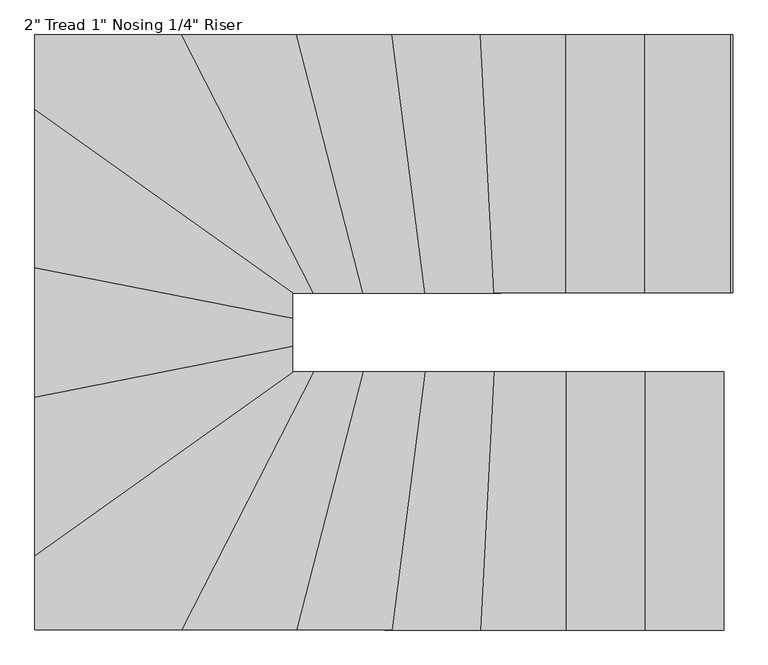
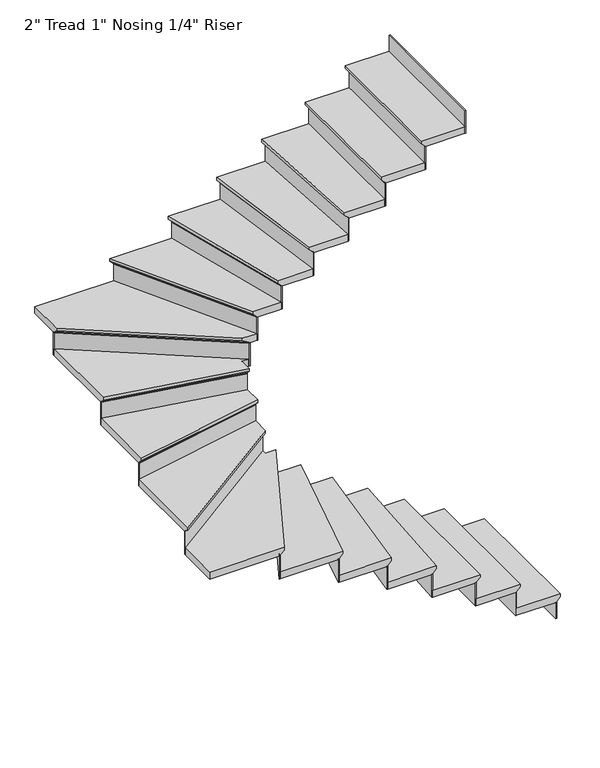
"""IFC4 building model written with IfcOpenShell, lengths in millimetres: stair flight geometry."""

from ifc_helpers import new_model, si_unit, origin, place, context, project, spatial, faceted_brep, source, transform, mapped, element, save


def stair_flight_62da4333(model_context):
    return source(origin(), model_context, "Body", "Brep", [
        faceted_brep([(-3425.4930658, -1479.646371, 150.2833333), (-3425.4930658, -1479.646371, 169.3333333), (-3425.4930658, -2394.046371, 169.3333333), (-3425.4930658, -2394.046371, 150.2833333), (-3450.8930658, -1479.646371, 124.8833333), (-3450.8930658, -2394.046371, 124.8833333), (-3730.2930658, -1479.646371, 169.3333333), (-3730.2930658, -2394.046371, 169.3333333), (-3450.8930658, -2394.046371, 118.5333333), (-3730.2930658, -2394.046371, 118.5333333), (-3730.2930658, -1479.646371, 118.5333333), (-3450.8930658, -1479.646371, 118.5333333)], [[[0, 1, 2, 3]], [[4, 0, 3, 5]], [[2, 1, 6, 7]], [[8, 9, 10, 11]], [[2, 7, 9, 8, 5, 3]], [[8, 11, 4, 5]], [[6, 1, 0, 4, 11, 10]], [[7, 6, 10, 9]]]),
        faceted_brep([(-3450.8930658, -1479.646371, 118.5333333), (-3450.8930658, -1479.646371, 0.0), (-3457.2430658, -1479.646371, 0.0), (-3457.2430658, -1479.646371, 118.5333333), (-3450.8930658, -2394.046371, 118.5333333), (-3457.2430658, -2394.046371, 118.5333333), (-3457.2430658, -2394.046371, 0.0), (-3450.8930658, -2394.046371, 0.0)], [[[0, 1, 2, 3]], [[4, 5, 6, 7]], [[1, 0, 4, 7]], [[2, 1, 7, 6]], [[3, 2, 6, 5]], [[0, 3, 5, 4]]]),
        faceted_brep([(-3730.2930658, -1479.646371, 287.8666667), (-3730.2930658, -1479.646371, 118.5333333), (-3736.6430658, -1479.646371, 118.5333333), (-3736.6430658, -1479.646371, 287.8666667), (-3730.2930658, -2394.046371, 287.8666667), (-3736.6430658, -2394.046371, 287.8666667), (-3736.6430658, -2394.046371, 118.5333333), (-3730.2930658, -2394.046371, 118.5333333)], [[[0, 1, 2, 3]], [[4, 5, 6, 7]], [[1, 0, 4, 7]], [[2, 1, 7, 6]], [[3, 2, 6, 5]], [[0, 3, 5, 4]]]),
        faceted_brep([(-3704.8930658, -2394.046371, 338.6666667), (-3704.8930658, -1479.646371, 338.6666667), (-4009.6930658, -1479.646371, 338.6666667), (-4009.6930658, -2394.046371, 338.6666667), (-3730.2930658, -2394.046371, 287.8666667), (-4009.6930658, -2394.046371, 287.8666667), (-4009.6930658, -1479.646371, 287.8666667), (-3730.2930658, -1479.646371, 287.8666667), (-3730.2930658, -2394.046371, 294.2166667), (-3704.8930658, -2394.046371, 319.6166667), (-3730.2930658, -1479.646371, 294.2166667), (-3704.8930658, -1479.646371, 319.6166667)], [[[0, 1, 2, 3]], [[4, 5, 6, 7]], [[0, 3, 5, 4, 8, 9]], [[4, 7, 10, 8]], [[2, 1, 11, 10, 7, 6]], [[3, 2, 6, 5]], [[11, 1, 0, 9]], [[10, 11, 9, 8]]]),
        faceted_brep([(-4009.6930658, -1479.646371, 457.2), (-4009.6930658, -1479.646371, 287.8666667), (-4016.0430658, -1479.646371, 287.8666667), (-4016.0430658, -1479.646371, 457.2), (-4009.6930658, -2394.046371, 457.2), (-4016.0430658, -2394.046371, 457.2), (-4016.0430658, -2394.046371, 287.8666667), (-4009.6930658, -2394.046371, 287.8666667)], [[[0, 1, 2, 3]], [[4, 5, 6, 7]], [[1, 0, 4, 7]], [[2, 1, 7, 6]], [[3, 2, 6, 5]], [[0, 3, 5, 4]]]),
        faceted_brep([(-3984.2930658, -2394.046371, 508.0), (-3984.2930658, -1479.646371, 508.0), (-4265.3602273, -1479.646371, 508.0), (-4312.8944977, -2394.046371, 508.0), (-4009.6930658, -2394.046371, 457.2), (-4312.8944977, -2394.046371, 457.2), (-4265.3602273, -1479.646371, 457.2), (-4009.6930658, -1479.646371, 457.2), (-4009.6930658, -2394.046371, 463.55), (-3984.2930658, -2394.046371, 488.95), (-4009.6930658, -1479.646371, 463.55), (-3984.2930658, -1479.646371, 488.95)], [[[0, 1, 2, 3]], [[4, 5, 6, 7]], [[0, 3, 5, 4, 8, 9]], [[4, 7, 10, 8]], [[2, 1, 11, 10, 7, 6]], [[3, 2, 6, 5]], [[11, 1, 0, 9]], [[10, 11, 9, 8]]]),
        faceted_brep([(-4265.3602273, -1479.646371, 626.5333333), (-4265.3602273, -1479.646371, 457.2), (-4271.7188014, -1479.646371, 457.2), (-4271.7188014, -1479.646371, 626.5333333), (-4312.8944977, -2394.046371, 626.5333333), (-4319.2530718, -2394.046371, 626.5333333), (-4319.2530718, -2394.046371, 457.2), (-4312.8944977, -2394.046371, 457.2)], [[[0, 1, 2, 3]], [[4, 5, 6, 7]], [[1, 0, 4, 7]], [[2, 1, 7, 6]], [[3, 2, 6, 5]], [[0, 3, 5, 4]]]),
        faceted_brep([(-4287.460201, -2394.046371, 677.3333333), (-4239.9259306, -1479.646371, 677.3333333), (-4509.5269271, -1479.646371, 677.3333333), (-4627.8829788, -2394.046371, 677.3333333), (-4312.8944977, -2394.046371, 626.5333333), (-4627.8829788, -2394.046371, 626.5333333), (-4509.5269271, -1479.646371, 626.5333333), (-4265.3602273, -1479.646371, 626.5333333), (-4312.8944977, -2394.046371, 632.8833333), (-4287.460201, -2394.046371, 658.2833333), (-4265.3602273, -1479.646371, 632.8833333), (-4239.9259306, -1479.646371, 658.2833333)], [[[0, 1, 2, 3]], [[4, 5, 6, 7]], [[0, 3, 5, 4, 8, 9]], [[4, 7, 10, 8]], [[2, 1, 11, 10, 7, 6]], [[3, 2, 6, 5]], [[11, 1, 0, 9]], [[10, 11, 9, 8]]]),
        faceted_brep([(-4509.5269271, -1479.646371, 795.8666667), (-4509.5269271, -1479.646371, 626.5333333), (-4515.9298989, -1479.646371, 626.5333333), (-4515.9298989, -1479.646371, 795.8666667), (-4627.8829788, -2394.046371, 795.8666667), (-4634.2859505, -2394.046371, 795.8666667), (-4634.2859505, -2394.046371, 626.5333333), (-4627.8829788, -2394.046371, 626.5333333)], [[[0, 1, 2, 3]], [[4, 5, 6, 7]], [[1, 0, 4, 7]], [[2, 1, 7, 6]], [[3, 2, 6, 5]], [[0, 3, 5, 4]]]),
        faceted_brep([(-4602.2710916, -2394.046371, 846.6666667), (-4483.91504, -1479.646371, 846.6666667), (-4731.1541496, -1479.646371, 846.6666667), (-4966.284597, -2394.046371, 846.6666667), (-4627.8829788, -2394.046371, 795.8666667), (-4966.284597, -2394.046371, 795.8666667), (-4731.1541496, -1479.646371, 795.8666667), (-4509.5269271, -1479.646371, 795.8666667), (-4627.8829788, -2394.046371, 802.2166667), (-4602.2710916, -2394.046371, 827.6166667), (-4509.5269271, -1479.646371, 802.2166667), (-4483.91504, -1479.646371, 827.6166667)], [[[0, 1, 2, 3]], [[4, 5, 6, 7]], [[0, 3, 5, 4, 8, 9]], [[4, 7, 10, 8]], [[2, 1, 11, 10, 7, 6]], [[3, 2, 6, 5]], [[11, 1, 0, 9]], [[10, 11, 9, 8]]]),
        faceted_brep([(-4731.1541496, -1479.646371, 965.2), (-4731.1541496, -1479.646371, 795.8666667), (-4737.7107264, -1479.646371, 795.8666667), (-4737.7107264, -1479.646371, 965.2), (-4966.284597, -2394.046371, 965.2), (-4972.8411738, -2394.046371, 965.2), (-4972.8411738, -2394.046371, 795.8666667), (-4966.284597, -2394.046371, 795.8666667)], [[[0, 1, 2, 3]], [[4, 5, 6, 7]], [[1, 0, 4, 7]], [[2, 1, 7, 6]], [[3, 2, 6, 5]], [[0, 3, 5, 4]]]),
        faceted_brep([(-4940.0582895, -2394.046371, 1016.0), (-4704.9278421, -1479.646371, 1016.0), (-4907.5007857, -1479.646371, 1016.0), (-5376.325407, -2394.046371, 1016.0), (-4966.284597, -2394.046371, 965.2), (-5376.325407, -2394.046371, 965.2), (-4907.5007857, -1479.646371, 965.2), (-4731.1541496, -1479.646371, 965.2), (-4966.284597, -2394.046371, 971.55), (-4940.0582895, -2394.046371, 996.95), (-4731.1541496, -1479.646371, 971.55), (-4704.9278421, -1479.646371, 996.95)], [[[0, 1, 2, 3]], [[4, 5, 6, 7]], [[0, 3, 5, 4, 8, 9]], [[4, 7, 10, 8]], [[2, 1, 11, 10, 7, 6]], [[3, 2, 6, 5]], [[11, 1, 0, 9]], [[10, 11, 9, 8]]]),
        faceted_brep([(-4907.5007857, -1479.646371, 1134.5333333), (-4907.5007857, -1479.646371, 965.2), (-4914.6367688, -1479.646371, 965.2), (-4914.6367688, -1479.646371, 1134.5333333), (-5376.325407, -2394.046371, 1134.5333333), (-5383.4613901, -2394.046371, 1134.5333333), (-5383.4613901, -2394.046371, 965.2), (-5376.325407, -2394.046371, 965.2)], [[[0, 1, 2, 3]], [[4, 5, 6, 7]], [[1, 0, 4, 7]], [[2, 1, 7, 6]], [[3, 2, 6, 5]], [[0, 3, 5, 4]]]),
        faceted_brep([(-5867.6247577, -2100.3652373, 1185.3333333), (-5867.6247577, -2394.046371, 1185.3333333), (-5347.7814744, -2394.046371, 1185.3333333), (-4878.9568531, -1479.646371, 1185.3333333), (-4953.2247577, -1479.646371, 1185.3333333), (-4953.2247577, -1450.0912881, 1185.3333333), (-5867.6247577, -2394.046371, 1134.5333333), (-5867.6247577, -2100.3652373, 1134.5333333), (-4953.2247577, -1450.0912881, 1134.5333333), (-4953.2247577, -1479.646371, 1134.5333333), (-4907.5007857, -1479.646371, 1134.5333333), (-5376.325407, -2394.046371, 1134.5333333), (-5376.325407, -2394.046371, 1140.8833333), (-5347.7814744, -2394.046371, 1166.2833333), (-4907.5007857, -1479.646371, 1140.8833333), (-4878.9568531, -1479.646371, 1166.2833333)], [[[0, 1, 2, 3, 4, 5]], [[6, 7, 8, 9, 10, 11]], [[1, 0, 7, 6]], [[2, 1, 6, 11, 12, 13]], [[11, 10, 14, 12]], [[4, 3, 15, 14, 10, 9]], [[5, 4, 9, 8]], [[0, 5, 8, 7]], [[15, 3, 2, 13]], [[14, 15, 13, 12]]]),
        faceted_brep([(-4953.2247577, -1450.0912881, 1303.8666667), (-4953.2247577, -1450.0912881, 1134.5333333), (-4953.2247577, -1442.2993133, 1134.5333333), (-4953.2247577, -1442.2993133, 1303.8666667), (-5867.6247577, -2100.3652373, 1303.8666667), (-5867.6247577, -2092.5732625, 1303.8666667), (-5867.6247577, -2092.5732625, 1134.5333333), (-5867.6247577, -2100.3652373, 1134.5333333)], [[[0, 1, 2, 3]], [[4, 5, 6, 7]], [[1, 0, 4, 7]], [[2, 1, 7, 6]], [[3, 2, 6, 5]], [[0, 3, 5, 4]]]),
        faceted_brep([(-5867.6247577, -2131.5331365, 1354.6666667), (-4953.2247577, -1481.2591873, 1354.6666667), (-4953.2247577, -1363.6372011, 1354.6666667), (-5867.6247577, -1543.8780574, 1354.6666667), (-5867.6247577, -2100.3652373, 1303.8666667), (-5867.6247577, -1543.8780574, 1303.8666667), (-4953.2247577, -1363.6372011, 1303.8666667), (-4953.2247577, -1450.0912881, 1303.8666667), (-5867.6247577, -2100.3652373, 1310.2166667), (-5867.6247577, -2131.5331365, 1335.6166667), (-4953.2247577, -1450.0912881, 1310.2166667), (-4953.2247577, -1481.2591873, 1335.6166667)], [[[0, 1, 2, 3]], [[4, 5, 6, 7]], [[0, 3, 5, 4, 8, 9]], [[4, 7, 10, 8]], [[2, 1, 11, 10, 7, 6]], [[3, 2, 6, 5]], [[11, 1, 0, 9]], [[10, 11, 9, 8]]]),
        faceted_brep([(-4953.2247577, -1363.6372011, 1473.2), (-4953.2247577, -1363.6372011, 1303.8666667), (-4953.2247577, -1357.1650156, 1303.8666667), (-4953.2247577, -1357.1650156, 1473.2), (-5867.6247577, -1543.8780574, 1473.2), (-5867.6247577, -1537.405872, 1473.2), (-5867.6247577, -1537.405872, 1303.8666667), (-5867.6247577, -1543.8780574, 1303.8666667)], [[[0, 1, 2, 3]], [[4, 5, 6, 7]], [[1, 0, 4, 7]], [[2, 1, 7, 6]], [[3, 2, 6, 5]], [[0, 3, 5, 4]]]),
        faceted_brep([(-5867.6247577, -1569.7667991, 1524.0), (-4953.2247577, -1389.5259428, 1524.0), (-4953.2247577, -1264.4780574, 1524.0), (-5867.6247577, -1084.2372011, 1524.0), (-5867.6247577, -1543.8780574, 1473.2), (-5867.6247577, -1084.2372011, 1473.2), (-4953.2247577, -1264.4780574, 1473.2), (-4953.2247577, -1363.6372011, 1473.2), (-5867.6247577, -1543.8780574, 1479.55), (-5867.6247577, -1569.7667991, 1504.95), (-4953.2247577, -1363.6372011, 1479.55), (-4953.2247577, -1389.5259428, 1504.95)], [[[0, 1, 2, 3]], [[4, 5, 6, 7]], [[0, 3, 5, 4, 8, 9]], [[4, 7, 10, 8]], [[2, 1, 11, 10, 7, 6]], [[3, 2, 6, 5]], [[11, 1, 0, 9]], [[10, 11, 9, 8]]]),
        faceted_brep([(-4953.2247577, -1264.4780574, 1642.5333333), (-4953.2247577, -1264.4780574, 1473.2), (-4953.2247577, -1258.005872, 1473.2), (-4953.2247577, -1258.005872, 1642.5333333), (-5867.6247577, -1084.2372011, 1642.5333333), (-5867.6247577, -1077.7650156, 1642.5333333), (-5867.6247577, -1077.7650156, 1473.2), (-5867.6247577, -1084.2372011, 1473.2)], [[[0, 1, 2, 3]], [[4, 5, 6, 7]], [[1, 0, 4, 7]], [[2, 1, 7, 6]], [[3, 2, 6, 5]], [[0, 3, 5, 4]]]),
        faceted_brep([(-5867.6247577, -1110.1259428, 1693.3333333), (-4953.2247577, -1290.3667991, 1693.3333333), (-4953.2247577, -1200.246371, 1693.3333333), (-4907.1292831, -1200.246371, 1693.3333333), (-5867.6247577, -517.1917063, 1693.3333333), (-5867.6247577, -1084.2372011, 1642.5333333), (-5867.6247577, -517.1917063, 1642.5333333), (-4907.1292831, -1200.246371, 1642.5333333), (-4953.2247577, -1200.246371, 1642.5333333), (-4953.2247577, -1264.4780574, 1642.5333333), (-5867.6247577, -1084.2372011, 1648.8833333), (-5867.6247577, -1110.1259428, 1674.2833333), (-4953.2247577, -1264.4780574, 1648.8833333), (-4953.2247577, -1290.3667991, 1674.2833333)], [[[0, 1, 2, 3, 4]], [[5, 6, 7, 8, 9]], [[0, 4, 6, 5, 10, 11]], [[5, 9, 12, 10]], [[2, 1, 13, 12, 9, 8]], [[3, 2, 8, 7]], [[4, 3, 7, 6]], [[13, 1, 0, 11]], [[12, 13, 11, 10]]]),
        faceted_brep([(-4907.1292831, -1200.246371, 1811.8666667), (-4907.1292831, -1200.246371, 1642.5333333), (-4896.1723907, -1200.246371, 1642.5333333), (-4896.1723907, -1200.246371, 1811.8666667), (-5867.6247577, -517.1917063, 1811.8666667), (-5867.6247577, -509.3997315, 1811.8666667), (-5867.6247577, -509.3997315, 1642.5333333), (-5867.6247577, -517.1917063, 1642.5333333)], [[[0, 1, 2, 3]], [[4, 5, 6, 7]], [[1, 0, 4, 7]], [[2, 1, 7, 6]], [[3, 2, 6, 5]], [[0, 3, 5, 4]]]),
        faceted_brep([(-5319.2375419, -285.846371, 1862.6666667), (-5867.6247577, -285.846371, 1862.6666667), (-5867.6247577, -548.3596055, 1862.6666667), (-4950.9568531, -1200.246371, 1862.6666667), (-4850.4129206, -1200.246371, 1862.6666667), (-5867.6247577, -285.846371, 1811.8666667), (-5319.2375419, -285.846371, 1811.8666667), (-4850.4129206, -1200.246371, 1811.8666667), (-4907.1292831, -1200.246371, 1811.8666667), (-5867.6247577, -517.1917063, 1811.8666667), (-5867.6247577, -517.1917063, 1818.2166667), (-5867.6247577, -548.3596055, 1843.6166667), (-4907.1292831, -1200.246371, 1818.2166667), (-4950.9568531, -1200.246371, 1843.6166667)], [[[0, 1, 2, 3, 4]], [[5, 6, 7, 8, 9]], [[1, 0, 6, 5]], [[2, 1, 5, 9, 10, 11]], [[9, 8, 12, 10]], [[4, 3, 13, 12, 8, 7]], [[0, 4, 7, 6]], [[13, 3, 2, 11]], [[12, 13, 11, 10]]]),
        faceted_brep([(-4850.4129206, -1200.246371, 1981.2), (-4850.4129206, -1200.246371, 1811.8666667), (-4843.2769375, -1200.246371, 1811.8666667), (-4843.2769375, -1200.246371, 1981.2), (-5319.2375419, -285.846371, 1981.2), (-5312.1015588, -285.846371, 1981.2), (-5312.1015588, -285.846371, 1811.8666667), (-5319.2375419, -285.846371, 1811.8666667)], [[[0, 1, 2, 3]], [[4, 5, 6, 7]], [[1, 0, 4, 7]], [[2, 1, 7, 6]], [[3, 2, 6, 5]], [[0, 3, 5, 4]]]),
        faceted_brep([(-5347.7814744, -285.846371, 2032.0), (-4878.9568531, -1200.246371, 2032.0), (-4678.7015346, -1200.246371, 2032.0), (-4913.831982, -285.846371, 2032.0), (-5319.2375419, -285.846371, 1981.2), (-4913.831982, -285.846371, 1981.2), (-4678.7015346, -1200.246371, 1981.2), (-4850.4129206, -1200.246371, 1981.2), (-5319.2375419, -285.846371, 1987.55), (-5347.7814744, -285.846371, 2012.95), (-4850.4129206, -1200.246371, 1987.55), (-4878.9568531, -1200.246371, 2012.95)], [[[0, 1, 2, 3]], [[4, 5, 6, 7]], [[0, 3, 5, 4, 8, 9]], [[4, 7, 10, 8]], [[2, 1, 11, 10, 7, 6]], [[3, 2, 6, 5]], [[11, 1, 0, 9]], [[10, 11, 9, 8]]]),
        faceted_brep([(-4678.7015346, -1200.246371, 2150.5333333), (-4678.7015346, -1200.246371, 1981.2), (-4672.1449578, -1200.246371, 1981.2), (-4672.1449578, -1200.246371, 2150.5333333), (-4913.831982, -285.846371, 2150.5333333), (-4907.2754052, -285.846371, 2150.5333333), (-4907.2754052, -285.846371, 1981.2), (-4913.831982, -285.846371, 1981.2)], [[[0, 1, 2, 3]], [[4, 5, 6, 7]], [[1, 0, 4, 7]], [[2, 1, 7, 6]], [[3, 2, 6, 5]], [[0, 3, 5, 4]]]),
        faceted_brep([(-4940.0582895, -285.846371, 2201.3333333), (-4704.9278421, -1200.246371, 2201.3333333), (-4458.3031529, -1200.246371, 2201.3333333), (-4576.6592045, -285.846371, 2201.3333333), (-4913.831982, -285.846371, 2150.5333333), (-4576.6592045, -285.846371, 2150.5333333), (-4458.3031529, -1200.246371, 2150.5333333), (-4678.7015346, -1200.246371, 2150.5333333), (-4913.831982, -285.846371, 2156.8833333), (-4940.0582895, -285.846371, 2182.2833333), (-4678.7015346, -1200.246371, 2156.8833333), (-4704.9278421, -1200.246371, 2182.2833333)], [[[0, 1, 2, 3]], [[4, 5, 6, 7]], [[0, 3, 5, 4, 8, 9]], [[4, 7, 10, 8]], [[2, 1, 11, 10, 7, 6]], [[3, 2, 6, 5]], [[11, 1, 0, 9]], [[10, 11, 9, 8]]]),
        faceted_brep([(-4458.3031529, -1200.246371, 2319.8666667), (-4458.3031529, -1200.246371, 2150.5333333), (-4451.9001811, -1200.246371, 2150.5333333), (-4451.9001811, -1200.246371, 2319.8666667), (-4576.6592045, -285.846371, 2319.8666667), (-4570.2562327, -285.846371, 2319.8666667), (-4570.2562327, -285.846371, 2150.5333333), (-4576.6592045, -285.846371, 2150.5333333)], [[[0, 1, 2, 3]], [[4, 5, 6, 7]], [[1, 0, 4, 7]], [[2, 1, 7, 6]], [[3, 2, 6, 5]], [[0, 3, 5, 4]]]),
        faceted_brep([(-4602.2710916, -285.846371, 2370.6666667), (-4483.91504, -1200.246371, 2370.6666667), (-4214.4916339, -1200.246371, 2370.6666667), (-4262.0259044, -285.846371, 2370.6666667), (-4576.6592045, -285.846371, 2319.8666667), (-4262.0259044, -285.846371, 2319.8666667), (-4214.4916339, -1200.246371, 2319.8666667), (-4458.3031529, -1200.246371, 2319.8666667), (-4576.6592045, -285.846371, 2326.2166667), (-4602.2710916, -285.846371, 2351.6166667), (-4458.3031529, -1200.246371, 2326.2166667), (-4483.91504, -1200.246371, 2351.6166667)], [[[0, 1, 2, 3]], [[4, 5, 6, 7]], [[0, 3, 5, 4, 8, 9]], [[4, 7, 10, 8]], [[2, 1, 11, 10, 7, 6]], [[3, 2, 6, 5]], [[11, 1, 0, 9]], [[10, 11, 9, 8]]]),
        faceted_brep([(-4214.4916339, -1200.246371, 2489.2), (-4214.4916339, -1200.246371, 2319.8666667), (-4208.1330598, -1200.246371, 2319.8666667), (-4208.1330598, -1200.246371, 2489.2), (-4262.0259044, -285.846371, 2489.2), (-4255.6673302, -285.846371, 2489.2), (-4255.6673302, -285.846371, 2319.8666667), (-4262.0259044, -285.846371, 2319.8666667)], [[[0, 1, 2, 3]], [[4, 5, 6, 7]], [[1, 0, 4, 7]], [[2, 1, 7, 6]], [[3, 2, 6, 5]], [[0, 3, 5, 4]]]),
        faceted_brep([(-4287.460201, -285.846371, 2540.0), (-4239.9259306, -1200.246371, 2540.0), (-3958.8930658, -1200.246371, 2540.0), (-3958.8930658, -285.846371, 2540.0), (-4262.0259044, -285.846371, 2489.2), (-3958.8930658, -285.846371, 2489.2), (-3958.8930658, -1200.246371, 2489.2), (-4214.4916339, -1200.246371, 2489.2), (-4262.0259044, -285.846371, 2495.55), (-4287.460201, -285.846371, 2520.95), (-4214.4916339, -1200.246371, 2495.55), (-4239.9259306, -1200.246371, 2520.95)], [[[0, 1, 2, 3]], [[4, 5, 6, 7]], [[0, 3, 5, 4, 8, 9]], [[4, 7, 10, 8]], [[2, 1, 11, 10, 7, 6]], [[3, 2, 6, 5]], [[11, 1, 0, 9]], [[10, 11, 9, 8]]]),
        faceted_brep([(-3958.8930658, -1200.246371, 2658.5333333), (-3958.8930658, -1200.246371, 2489.2), (-3952.5430658, -1200.246371, 2489.2), (-3952.5430658, -1200.246371, 2658.5333333), (-3958.8930658, -285.846371, 2658.5333333), (-3952.5430658, -285.846371, 2658.5333333), (-3952.5430658, -285.846371, 2489.2), (-3958.8930658, -285.846371, 2489.2)], [[[0, 1, 2, 3]], [[4, 5, 6, 7]], [[1, 0, 4, 7]], [[2, 1, 7, 6]], [[3, 2, 6, 5]], [[0, 3, 5, 4]]]),
        faceted_brep([(-3984.2930658, -285.846371, 2709.3333333), (-3984.2930658, -1200.246371, 2709.3333333), (-3679.4930658, -1200.246371, 2709.3333333), (-3679.4930658, -285.846371, 2709.3333333), (-3958.8930658, -285.846371, 2658.5333333), (-3679.4930658, -285.846371, 2658.5333333), (-3679.4930658, -1200.246371, 2658.5333333), (-3958.8930658, -1200.246371, 2658.5333333), (-3958.8930658, -285.846371, 2664.8833333), (-3984.2930658, -285.846371, 2690.2833333), (-3958.8930658, -1200.246371, 2664.8833333), (-3984.2930658, -1200.246371, 2690.2833333)], [[[0, 1, 2, 3]], [[4, 5, 6, 7]], [[0, 3, 5, 4, 8, 9]], [[4, 7, 10, 8]], [[2, 1, 11, 10, 7, 6]], [[3, 2, 6, 5]], [[11, 1, 0, 9]], [[10, 11, 9, 8]]]),
        faceted_brep([(-3679.4930658, -1200.246371, 2827.8666667), (-3679.4930658, -1200.246371, 2658.5333333), (-3673.1430658, -1200.246371, 2658.5333333), (-3673.1430658, -1200.246371, 2827.8666667), (-3679.4930658, -285.846371, 2827.8666667), (-3673.1430658, -285.846371, 2827.8666667), (-3673.1430658, -285.846371, 2658.5333333), (-3679.4930658, -285.846371, 2658.5333333)], [[[0, 1, 2, 3]], [[4, 5, 6, 7]], [[1, 0, 4, 7]], [[2, 1, 7, 6]], [[3, 2, 6, 5]], [[0, 3, 5, 4]]]),
        faceted_brep([(-3400.0930658, -1200.246371, 2997.2), (-3400.0930658, -1200.246371, 2827.8666667), (-3393.7430658, -1200.246371, 2827.8666667), (-3393.7430658, -1200.246371, 2997.2), (-3400.0930658, -285.846371, 2997.2), (-3393.7430658, -285.846371, 2997.2), (-3393.7430658, -285.846371, 2827.8666667), (-3400.0930658, -285.846371, 2827.8666667)], [[[0, 1, 2, 3]], [[4, 5, 6, 7]], [[1, 0, 4, 7]], [[2, 1, 7, 6]], [[3, 2, 6, 5]], [[0, 3, 5, 4]]]),
        faceted_brep([(-3704.8930658, -285.846371, 2878.6666667), (-3704.8930658, -1200.246371, 2878.6666667), (-3400.0930658, -1200.246371, 2878.6666667), (-3400.0930658, -285.846371, 2878.6666667), (-3679.4930658, -285.846371, 2827.8666667), (-3400.0930658, -285.846371, 2827.8666667), (-3400.0930658, -1200.246371, 2827.8666667), (-3679.4930658, -1200.246371, 2827.8666667), (-3679.4930658, -285.846371, 2834.2166667), (-3704.8930658, -285.846371, 2859.6166667), (-3679.4930658, -1200.246371, 2834.2166667), (-3704.8930658, -1200.246371, 2859.6166667)], [[[0, 1, 2, 3]], [[4, 5, 6, 7]], [[0, 3, 5, 4, 8, 9]], [[4, 7, 10, 8]], [[2, 1, 11, 10, 7, 6]], [[3, 2, 6, 5]], [[11, 1, 0, 9]], [[10, 11, 9, 8]]]),
    ])


if __name__ == "__main__":
    model = new_model("IFC4")
    model_context = context("Model", 3, world=origin())
    ifc_project = project(units=[si_unit("LENGTHUNIT", "METRE", prefix="MILLI")], contexts=[model_context])
    site = spatial("IfcSite", under=ifc_project)
    building = spatial("IfcBuilding", under=site)
    placement = place(None, origin())
    stair_flight_shape = stair_flight_62da4333(model_context)
    element("IfcStairFlight", 1, ObjectType="2\" Tread 1\" Nosing 1/4\" Riser", at=placement, inside=building, context=model_context, shape_type="MappedRepresentation", body=[
        mapped(stair_flight_shape, transform((0.0, 0.0, 0.0), x_axis=(1.0, 0.0, 0.0), y_axis=(0.0, 1.0, 0.0), z_axis=(0.0, 0.0, 1.0))),
    ])
    save(model, "model.ifc")
